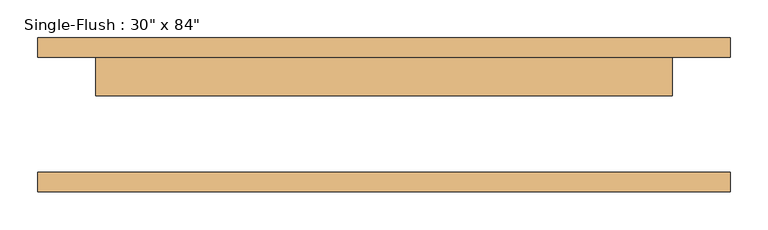
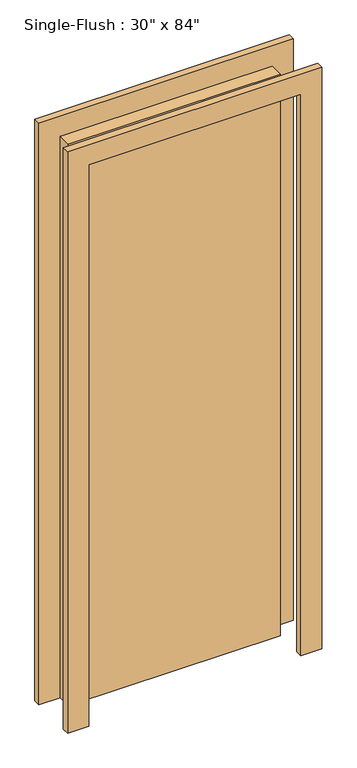
"""IFC4 building model written with IfcOpenShell, lengths in millimetres: door geometry."""

from ifc_helpers import new_model, si_unit, frame, origin, origin_with_axes, place, context, project, spatial, polyline, outline, extrude, source, transform, mapped, element, save


def door_a9addea7(model_context):
    return source(origin(), model_context, "Body", "SweptSolid", [
        extrude(outline(polyline([(2209.8, -457.2), (0.0, -457.2), (0.0, -381.0), (2133.6, -381.0), (2133.6, 381.0), (0.0, 381.0), (0.0, 457.2), (2209.8, 457.2), (2209.8, -457.2)])), frame((0.0, 76.2, 0.0), z_axis=(0.0, 1.0, 0.0), x_axis=(0.0, 0.0, 1.0)), (0.0, 0.0, 1.0), 25.4),
        extrude(outline(polyline([(2209.8, 457.2), (2209.8, -457.2), (0.0, -457.2), (0.0, -381.0), (2133.6, -381.0), (2133.6, 381.0), (0.0, 381.0), (0.0, 457.2), (2209.8, 457.2)])), frame((0.0, -101.6, 0.0), z_axis=(0.0, 1.0, 0.0), x_axis=(0.0, 0.0, 1.0)), (0.0, 0.0, 1.0), 25.4),
        extrude(outline(polyline([(381.0, 25.4), (-381.0, 25.4), (-381.0, 76.2), (381.0, 76.2), (381.0, 25.4)])), origin_with_axes(), (0.0, 0.0, 1.0), 2133.6),
    ])


if __name__ == "__main__":
    model = new_model("IFC4")
    model_context = context("Model", 3, world=origin())
    ifc_project = project(units=[si_unit("LENGTHUNIT", "METRE", prefix="MILLI")], contexts=[model_context])
    site = spatial("IfcSite", under=ifc_project)
    building = spatial("IfcBuilding", under=site)
    placement = place(None, origin())
    door_shape = door_a9addea7(model_context)
    element("IfcDoor", 1, ObjectType="Single-Flush : 30\" x 84\"", at=placement, inside=building, context=model_context, shape_type="MappedRepresentation", body=[
        mapped(door_shape, transform((0.0, 0.0, 0.0), x_axis=(1.0, 0.0, 0.0), y_axis=(0.0, 1.0, 0.0), z_axis=(0.0, 0.0, 1.0))),
    ])
    save(model, "model.ifc")

# Revit data of these elements
# Type "Single-Flush : 30\" x 84\""
#   Type Mark = "4"
#   Construction Type Id = "MDOOR"
#   Assembly Code = "C1020"
#   Analytic Construction = "Metal"
#   Thickness = 0' - 2"
#   Heat Transfer Coefficient (U) = 0.651978 BTU/(h·ft²·°F)
#   Height = 7' - 0"
#   Trim Projection Ext = 0' - 1"
#   Trim Projection Int = 0' - 1"
#   Trim Width = 0' - 3"
#   Width = 2' - 6"
#   Define Thermal Properties by = 1
#   Door Material = Door - Panel
#   Frame Material = Door - Frame
#   Visual Light Transmittance = 0
#   Solar Heat Gain Coefficient = 0
#   Function = (empty or 0)
#   Wall Closure = (empty or 0)
# Element 1 (IfcDoor, "Single-Flush : 30\" x 84\"")
#   Materials on its faces: "Door - Frame", "Door - Panel"
# Materials
#   "Door - Panel": class "Wood", colour RGB 210 159 95, transparency 0
#   "Door - Frame": colour RGB 118 70 51, transparency 0
